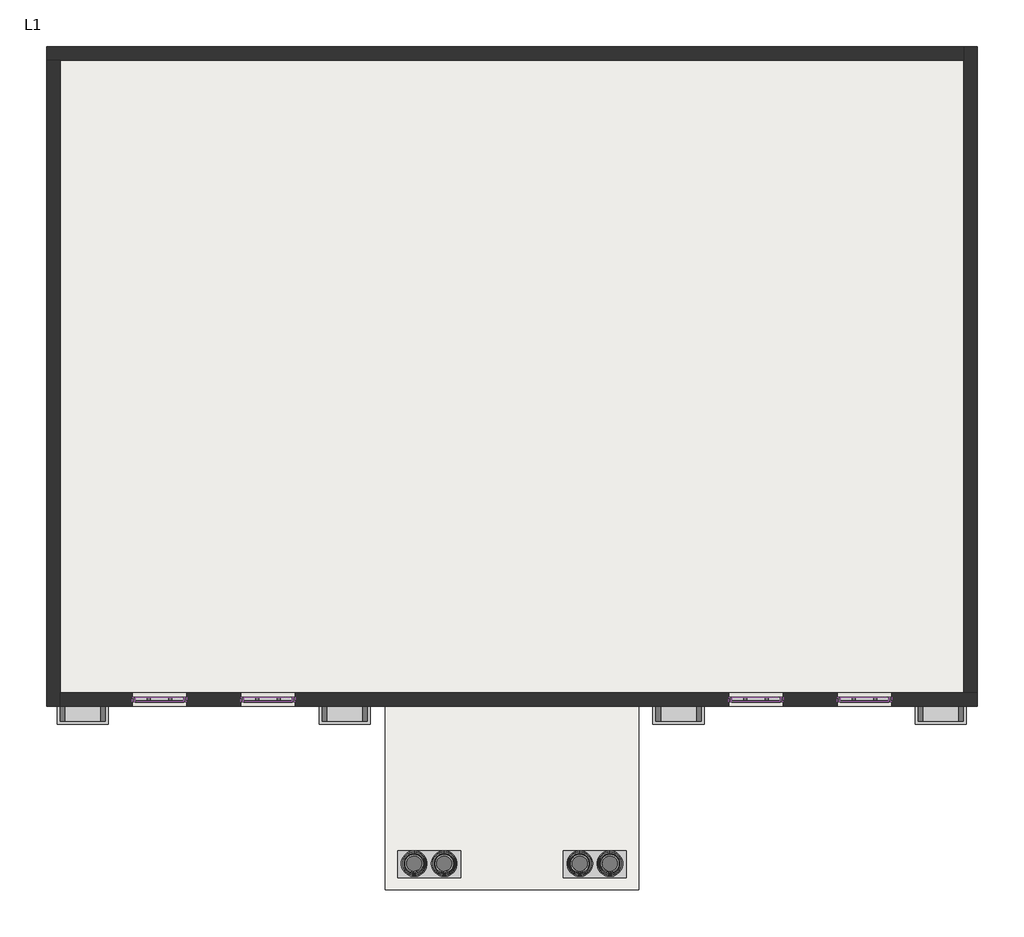
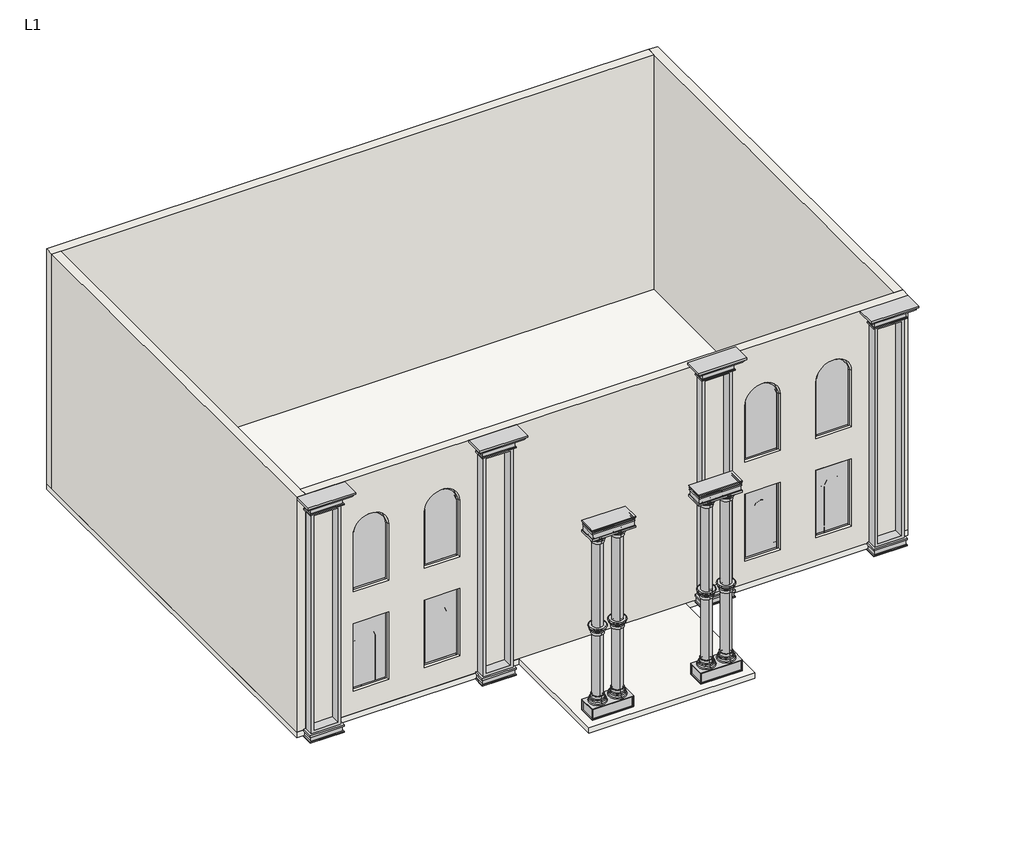
# One storey: 32 members, 10 proxies, 4 walls, 1 plate, 1 slab.
"""IFC4 building model written with IfcOpenShell, lengths in millimetres."""

from ifc_helpers import new_model, si_unit, frame, origin, place, context, project, spatial, polyline, circle_curve, outline, extrude, faceted_brep, transform, mapped, element, save
from ifc_brep_helpers import plane_surface, revolved_surface, advanced_brep
from components import generic_models_10_generic_models_9_50d809b8, generic_models_12_generic_models_12_08b21b51, generic_models_14_generic_models_14_9f9ef7df, generic_models_14_generic_models_14_a82bafd3, generic_models_14_generic_models_14_26f09abb, generic_models_5_generic_models_1_f7cfe2cb, member_492a078d, member_19d0c1c6, member_fb5b44a5, member_86f0261c, system_panel_glazed_d30904ce

model = new_model("IFC4")

# Units and contexts
model_context = context("Model", 3, world=origin())
ifc_project = project(units=[si_unit("LENGTHUNIT", "METRE", prefix="MILLI")], contexts=[model_context])

# Site, building, storey
site = spatial("IfcSite", under=ifc_project)
building = spatial("IfcBuilding", under=site)
storey = spatial("IfcBuildingStorey", under=building, Name="L1", Elevation=0.0)

# Proxies
placement = place(None, origin())
generic_models_10_generic_models_9_shape = generic_models_10_generic_models_9_50d809b8(model_context)
element("IfcBuildingElementProxy", 1, Name="Generic Models 10 : Generic Models 9", ObjectType="Generic Models 10 : Generic Models 9", at=placement, inside=storey, context=model_context, shape_type="MappedRepresentation", body=[
    mapped(generic_models_10_generic_models_9_shape, transform((14467.7065642, 0.0, 0.0), x_axis=(1.0, 0.0, 0.0), y_axis=(0.0, 1.0, 0.0), z_axis=(0.0, 0.0, 1.0))),
])
element("IfcBuildingElementProxy", 2, Name="Generic Models 11 : Generic Models 9", ObjectType="Generic Models 11 : Generic Models 9", at=placement, inside=storey, context=model_context, shape_type="MappedRepresentation", body=[
    mapped(generic_models_10_generic_models_9_shape, transform((4419.6, 0.0, 0.0), x_axis=(1.0, 0.0, 0.0), y_axis=(0.0, 1.0, 0.0), z_axis=(0.0, 0.0, 1.0))),
])
generic_models_12_generic_models_12_shape = generic_models_12_generic_models_12_08b21b51(model_context)
element("IfcBuildingElementProxy", 3, Name="Generic Models 12 : Generic Models 12", ObjectType="Generic Models 12 : Generic Models 12", at=placement, inside=storey, context=model_context, shape_type="MappedRepresentation", body=[
    mapped(generic_models_12_generic_models_12_shape, transform((0.0, 0.0, 0.0), x_axis=(1.0, 0.0, 0.0), y_axis=(0.0, 1.0, 0.0), z_axis=(0.0, 0.0, 1.0))),
])
element("IfcBuildingElementProxy", 4, Name="Generic Models 13 : Generic Models 9", ObjectType="Generic Models 13 : Generic Models 9", at=placement, inside=storey, context=model_context, shape_type="MappedRepresentation", body=[
    mapped(generic_models_10_generic_models_9_shape, transform((10048.1065642, 0.0, 138.370057), x_axis=(1.0, 0.0, 0.0), y_axis=(0.0, 1.0, 0.0), z_axis=(0.0, 0.0, 1.0))),
])
generic_models_14_generic_models_14_shape = generic_models_14_generic_models_14_9f9ef7df(model_context)
generic_models_14_generic_models_14_2_shape = generic_models_14_generic_models_14_a82bafd3(model_context)
generic_models_14_generic_models_14_3_shape = generic_models_14_generic_models_14_26f09abb(model_context)
element("IfcBuildingElementProxy", 5, Name="Generic Models 14 : Generic Models 14", ObjectType="Generic Models 14 : Generic Models 14", at=placement, inside=storey, context=model_context, shape_type="MappedRepresentation", body=[
    mapped(generic_models_14_generic_models_14_shape, transform((0.0, 0.0, 0.0), x_axis=(1.0, 0.0, 0.0), y_axis=(0.0, 1.0, 0.0), z_axis=(0.0, 0.0, 1.0))),
    mapped(generic_models_14_generic_models_14_2_shape, transform((0.0, 0.0, 0.0), x_axis=(1.0, 0.0, 0.0), y_axis=(0.0, 1.0, 0.0), z_axis=(0.0, 0.0, 1.0))),
    mapped(generic_models_14_generic_models_14_3_shape, transform((0.0, 0.0, 0.0), x_axis=(1.0, 0.0, 0.0), y_axis=(0.0, 1.0, 0.0), z_axis=(0.0, 0.0, 1.0))),
])
generic_models_5_generic_models_1_shape = generic_models_5_generic_models_1_f7cfe2cb(model_context)
element("IfcBuildingElementProxy", 6, Name="Generic Models 5 : Generic Models 1", ObjectType="Generic Models 5 : Generic Models 1", at=placement, inside=storey, context=model_context, shape_type="MappedRepresentation", body=[
    mapped(generic_models_5_generic_models_1_shape, transform((0.0, 0.0, 0.0), x_axis=(1.0, 0.0, 0.0), y_axis=(0.0, 1.0, 0.0), z_axis=(0.0, 0.0, 1.0))),
])
element("IfcBuildingElementProxy", 7, Name="Generic Models 6 : Generic Models 1", ObjectType="Generic Models 6 : Generic Models 1", at=placement, inside=storey, context=model_context, shape_type="MappedRepresentation", body=[
    mapped(generic_models_5_generic_models_1_shape, transform((1828.8, 0.0, 0.0), x_axis=(1.0, 0.0, 0.0), y_axis=(0.0, 1.0, 0.0), z_axis=(0.0, 0.0, 1.0))),
])
element("IfcBuildingElementProxy", 8, Name="Generic Models 7 : Generic Models 1", ObjectType="Generic Models 7 : Generic Models 1", at=placement, inside=storey, context=model_context, shape_type="MappedRepresentation", body=[
    mapped(generic_models_5_generic_models_1_shape, transform((10058.4, 0.0, 0.0), x_axis=(1.0, 0.0, 0.0), y_axis=(0.0, 1.0, 0.0), z_axis=(0.0, 0.0, 1.0))),
])
element("IfcBuildingElementProxy", 9, Name="Generic Models 8 : Generic Models 1", ObjectType="Generic Models 8 : Generic Models 1", at=placement, inside=storey, context=model_context, shape_type="MappedRepresentation", body=[
    mapped(generic_models_5_generic_models_1_shape, transform((11887.2, 0.0, 0.0), x_axis=(1.0, 0.0, 0.0), y_axis=(0.0, 1.0, 0.0), z_axis=(0.0, 0.0, 1.0))),
])
element("IfcBuildingElementProxy", 10, Name="Generic Models 9 : Generic Models 9", ObjectType="Generic Models 9 : Generic Models 9", at=placement, inside=storey, context=model_context, shape_type="MappedRepresentation", body=[
    mapped(generic_models_10_generic_models_9_shape, transform((0.0, 0.0, 0.0), x_axis=(1.0, 0.0, 0.0), y_axis=(0.0, 1.0, 0.0), z_axis=(0.0, 0.0, 1.0))),
])

# Members
member_shape = member_492a078d(model_context)
element("IfcMember", 11, ObjectType="Rectangular Mullion : 2.5\" x 5\" rectangular", at=placement, inside=storey, context=model_context, shape_type="MappedRepresentation", body=[
    mapped(member_shape, transform((-6449.8825076, -4772.1608295, 3302.0), x_axis=(0.0, 0.0, -1.0), y_axis=(0.0, 1.0, 0.0), z_axis=(1.0, 0.0, 0.0))),
])
element("IfcMember", 12, ObjectType="Rectangular Mullion : 2.5\" x 5\" rectangular", at=placement, inside=storey, context=model_context, shape_type="MappedRepresentation", body=[
    mapped(member_shape, transform((-6449.8825076, -4772.1608295, 609.6), x_axis=(0.0, 0.0, -1.0), y_axis=(0.0, 1.0, 0.0), z_axis=(1.0, 0.0, 0.0))),
])
element("IfcMember", 13, ObjectType="Rectangular Mullion : 2.5\" x 5\" rectangular", at=placement, inside=storey, context=model_context, shape_type="MappedRepresentation", body=[
    mapped(member_shape, transform((-4621.0825076, -4772.1608295, 3302.0), x_axis=(0.0, 0.0, -1.0), y_axis=(0.0, 1.0, 0.0), z_axis=(1.0, 0.0, 0.0))),
])
element("IfcMember", 14, ObjectType="Rectangular Mullion : 2.5\" x 5\" rectangular", at=placement, inside=storey, context=model_context, shape_type="MappedRepresentation", body=[
    mapped(member_shape, transform((-4621.0825076, -4772.1608295, 609.6), x_axis=(0.0, 0.0, -1.0), y_axis=(0.0, 1.0, 0.0), z_axis=(1.0, 0.0, 0.0))),
])
element("IfcMember", 15, ObjectType="Rectangular Mullion : 2.5\" x 5\" rectangular", at=placement, inside=storey, context=model_context, shape_type="MappedRepresentation", body=[
    mapped(member_shape, transform((3608.5174924, -4772.1608295, 3302.0), x_axis=(0.0, 0.0, -1.0), y_axis=(0.0, 1.0, 0.0), z_axis=(1.0, 0.0, 0.0))),
])
element("IfcMember", 16, ObjectType="Rectangular Mullion : 2.5\" x 5\" rectangular", at=placement, inside=storey, context=model_context, shape_type="MappedRepresentation", body=[
    mapped(member_shape, transform((3608.5174924, -4772.1608295, 609.6), x_axis=(0.0, 0.0, -1.0), y_axis=(0.0, 1.0, 0.0), z_axis=(1.0, 0.0, 0.0))),
])
element("IfcMember", 17, ObjectType="Rectangular Mullion : 2.5\" x 5\" rectangular", at=placement, inside=storey, context=model_context, shape_type="MappedRepresentation", body=[
    mapped(member_shape, transform((5437.3174924, -4772.1608295, 3302.0), x_axis=(0.0, 0.0, -1.0), y_axis=(0.0, 1.0, 0.0), z_axis=(1.0, 0.0, 0.0))),
])
element("IfcMember", 18, ObjectType="Rectangular Mullion : 2.5\" x 5\" rectangular", at=placement, inside=storey, context=model_context, shape_type="MappedRepresentation", body=[
    mapped(member_shape, transform((5437.3174924, -4772.1608295, 609.6), x_axis=(0.0, 0.0, -1.0), y_axis=(0.0, 1.0, 0.0), z_axis=(1.0, 0.0, 0.0))),
])
member_2_shape = member_19d0c1c6(model_context)
element("IfcMember", 19, ObjectType="Rectangular Mullion : 2.5\" x 5\" rectangular", at=placement, inside=storey, context=model_context, shape_type="MappedRepresentation", body=[
    mapped(member_2_shape, transform((-6399.0825076, -4772.1608295, 4826.0), x_axis=(1.0, 0.0, 0.0), y_axis=(0.0, 1.0, 0.0), z_axis=(0.0, 0.0, 1.0))),
])
element("IfcMember", 20, ObjectType="Rectangular Mullion : 2.5\" x 5\" rectangular", at=placement, inside=storey, context=model_context, shape_type="MappedRepresentation", body=[
    mapped(member_2_shape, transform((-4570.2825076, -4772.1608295, 4826.0), x_axis=(1.0, 0.0, 0.0), y_axis=(0.0, 1.0, 0.0), z_axis=(0.0, 0.0, 1.0))),
])
element("IfcMember", 21, ObjectType="Rectangular Mullion : 2.5\" x 5\" rectangular", at=placement, inside=storey, context=model_context, shape_type="MappedRepresentation", body=[
    mapped(member_2_shape, transform((3659.3174924, -4772.1608295, 4826.0), x_axis=(1.0, 0.0, 0.0), y_axis=(0.0, 1.0, 0.0), z_axis=(0.0, 0.0, 1.0))),
])
element("IfcMember", 22, ObjectType="Rectangular Mullion : 2.5\" x 5\" rectangular", at=placement, inside=storey, context=model_context, shape_type="MappedRepresentation", body=[
    mapped(member_2_shape, transform((5488.1174924, -4772.1608295, 4826.0), x_axis=(1.0, 0.0, 0.0), y_axis=(0.0, 1.0, 0.0), z_axis=(0.0, 0.0, 1.0))),
])
member_3_shape = member_fb5b44a5(model_context)
element("IfcMember", 23, ObjectType="Rectangular Mullion : 2.5\" x 5\" rectangular", at=placement, inside=storey, context=model_context, shape_type="MappedRepresentation", body=[
    mapped(member_3_shape, transform((-7313.4825076, -4772.1608295, 4826.0), x_axis=(-1.0, 0.0, 0.0), y_axis=(0.0, 1.0, 0.0), z_axis=(0.0, 0.0, -1.0))),
])
element("IfcMember", 24, ObjectType="Rectangular Mullion : 2.5\" x 5\" rectangular", at=placement, inside=storey, context=model_context, shape_type="MappedRepresentation", body=[
    mapped(member_3_shape, transform((-5484.6825076, -4772.1608295, 4826.0), x_axis=(-1.0, 0.0, 0.0), y_axis=(0.0, 1.0, 0.0), z_axis=(0.0, 0.0, -1.0))),
])
element("IfcMember", 25, ObjectType="Rectangular Mullion : 2.5\" x 5\" rectangular", at=placement, inside=storey, context=model_context, shape_type="MappedRepresentation", body=[
    mapped(member_3_shape, transform((2744.9174924, -4772.1608295, 4826.0), x_axis=(-1.0, 0.0, 0.0), y_axis=(0.0, 1.0, 0.0), z_axis=(0.0, 0.0, -1.0))),
])
element("IfcMember", 26, ObjectType="Rectangular Mullion : 2.5\" x 5\" rectangular", at=placement, inside=storey, context=model_context, shape_type="MappedRepresentation", body=[
    mapped(member_3_shape, transform((4573.7174924, -4772.1608295, 4826.0), x_axis=(-1.0, 0.0, 0.0), y_axis=(0.0, 1.0, 0.0), z_axis=(0.0, 0.0, -1.0))),
])
element("IfcMember", 27, ObjectType="Rectangular Mullion : 2.5\" x 5\" rectangular", at=placement, inside=storey, context=model_context, shape_type="MappedRepresentation", body=[
    mapped(member_shape, transform((-7262.6825076, -4772.1608295, 2438.4), x_axis=(0.0, 0.0, 1.0), y_axis=(0.0, 1.0, 0.0), z_axis=(-1.0, 0.0, 0.0))),
])
element("IfcMember", 28, ObjectType="Rectangular Mullion : 2.5\" x 5\" rectangular", at=placement, inside=storey, context=model_context, shape_type="MappedRepresentation", body=[
    mapped(member_shape, transform((-5433.8825076, -4772.1608295, 2438.4), x_axis=(0.0, 0.0, 1.0), y_axis=(0.0, 1.0, 0.0), z_axis=(-1.0, 0.0, 0.0))),
])
element("IfcMember", 29, ObjectType="Rectangular Mullion : 2.5\" x 5\" rectangular", at=placement, inside=storey, context=model_context, shape_type="MappedRepresentation", body=[
    mapped(member_shape, transform((2795.7174924, -4772.1608295, 2438.4), x_axis=(0.0, 0.0, 1.0), y_axis=(0.0, 1.0, 0.0), z_axis=(-1.0, 0.0, 0.0))),
])
element("IfcMember", 30, ObjectType="Rectangular Mullion : 2.5\" x 5\" rectangular", at=placement, inside=storey, context=model_context, shape_type="MappedRepresentation", body=[
    mapped(member_shape, transform((4624.5174924, -4772.1608295, 2438.4), x_axis=(0.0, 0.0, 1.0), y_axis=(0.0, 1.0, 0.0), z_axis=(-1.0, 0.0, 0.0))),
])
element("IfcMember", 31, ObjectType="Rectangular Mullion : 2.5\" x 5\" rectangular", at=placement, inside=storey, context=model_context, shape_type="MappedRepresentation", body=[
    mapped(member_2_shape, transform((-7313.4825076, -4772.1608295, 3302.0), x_axis=(-1.0, 0.0, 0.0), y_axis=(0.0, 1.0, 0.0), z_axis=(0.0, 0.0, -1.0))),
])
element("IfcMember", 32, ObjectType="Rectangular Mullion : 2.5\" x 5\" rectangular", at=placement, inside=storey, context=model_context, shape_type="MappedRepresentation", body=[
    mapped(member_2_shape, transform((-5484.6825076, -4772.1608295, 3302.0), x_axis=(-1.0, 0.0, 0.0), y_axis=(0.0, 1.0, 0.0), z_axis=(0.0, 0.0, -1.0))),
])
element("IfcMember", 33, ObjectType="Rectangular Mullion : 2.5\" x 5\" rectangular", at=placement, inside=storey, context=model_context, shape_type="MappedRepresentation", body=[
    mapped(member_2_shape, transform((2744.9174924, -4772.1608295, 3302.0), x_axis=(-1.0, 0.0, 0.0), y_axis=(0.0, 1.0, 0.0), z_axis=(0.0, 0.0, -1.0))),
])
element("IfcMember", 34, ObjectType="Rectangular Mullion : 2.5\" x 5\" rectangular", at=placement, inside=storey, context=model_context, shape_type="MappedRepresentation", body=[
    mapped(member_2_shape, transform((4573.7174924, -4772.1608295, 3302.0), x_axis=(-1.0, 0.0, 0.0), y_axis=(0.0, 1.0, 0.0), z_axis=(0.0, 0.0, -1.0))),
])
member_4_shape = member_86f0261c(model_context)
element("IfcMember", 35, ObjectType="Rectangular Mullion : 2.5\" x 5\" rectangular", at=placement, inside=storey, context=model_context, shape_type="MappedRepresentation", body=[
    mapped(member_4_shape, transform((-7313.4825076, -4772.1608295, 609.6), x_axis=(-1.0, 0.0, 0.0), y_axis=(0.0, 1.0, 0.0), z_axis=(0.0, 0.0, -1.0))),
])
element("IfcMember", 36, ObjectType="Rectangular Mullion : 2.5\" x 5\" rectangular", at=placement, inside=storey, context=model_context, shape_type="MappedRepresentation", body=[
    mapped(member_4_shape, transform((-5484.6825076, -4772.1608295, 609.6), x_axis=(-1.0, 0.0, 0.0), y_axis=(0.0, 1.0, 0.0), z_axis=(0.0, 0.0, -1.0))),
])
element("IfcMember", 37, ObjectType="Rectangular Mullion : 2.5\" x 5\" rectangular", at=placement, inside=storey, context=model_context, shape_type="MappedRepresentation", body=[
    mapped(member_4_shape, transform((2744.9174924, -4772.1608295, 609.6), x_axis=(-1.0, 0.0, 0.0), y_axis=(0.0, 1.0, 0.0), z_axis=(0.0, 0.0, -1.0))),
])
element("IfcMember", 38, ObjectType="Rectangular Mullion : 2.5\" x 5\" rectangular", at=placement, inside=storey, context=model_context, shape_type="MappedRepresentation", body=[
    mapped(member_4_shape, transform((4573.7174924, -4772.1608295, 609.6), x_axis=(-1.0, 0.0, 0.0), y_axis=(0.0, 1.0, 0.0), z_axis=(0.0, 0.0, -1.0))),
])
element("IfcMember", 39, ObjectType="Rectangular Mullion : 2.5\" x 5\" rectangular", at=placement, inside=storey, context=model_context, shape_type="MappedRepresentation", body=[
    mapped(member_4_shape, transform((-6399.0825076, -4772.1608295, 2438.4), x_axis=(1.0, 0.0, 0.0), y_axis=(0.0, 1.0, 0.0), z_axis=(0.0, 0.0, 1.0))),
])
element("IfcMember", 40, ObjectType="Rectangular Mullion : 2.5\" x 5\" rectangular", at=placement, inside=storey, context=model_context, shape_type="MappedRepresentation", body=[
    mapped(member_4_shape, transform((-4570.2825076, -4772.1608295, 2438.4), x_axis=(1.0, 0.0, 0.0), y_axis=(0.0, 1.0, 0.0), z_axis=(0.0, 0.0, 1.0))),
])
element("IfcMember", 41, ObjectType="Rectangular Mullion : 2.5\" x 5\" rectangular", at=placement, inside=storey, context=model_context, shape_type="MappedRepresentation", body=[
    mapped(member_4_shape, transform((3659.3174924, -4772.1608295, 2438.4), x_axis=(1.0, 0.0, 0.0), y_axis=(0.0, 1.0, 0.0), z_axis=(0.0, 0.0, 1.0))),
])
element("IfcMember", 42, ObjectType="Rectangular Mullion : 2.5\" x 5\" rectangular", at=placement, inside=storey, context=model_context, shape_type="MappedRepresentation", body=[
    mapped(member_4_shape, transform((5488.1174924, -4772.1608295, 2438.4), x_axis=(1.0, 0.0, 0.0), y_axis=(0.0, 1.0, 0.0), z_axis=(0.0, 0.0, 1.0))),
])

# Plate
system_panel_glazed_shape = system_panel_glazed_d30904ce(model_context)
element("IfcPlate", 43, ObjectType="System Panel : Glazed", at=placement, inside=storey, context=model_context, shape_type="MappedRepresentation", body=[
    mapped(system_panel_glazed_shape, transform((-912.6825076, -4772.1608295, 660.4), x_axis=(-1.0, 0.0, 0.0), y_axis=(0.0, -1.0, 0.0), z_axis=(0.0, 0.0, 1.0))),
])

# Slab
element("IfcSlab", 44, ObjectType="6\"", at=placement, inside=storey, context=model_context, shape_type="SweptSolid", body=[
    extrude(outline(polyline([(6935.9174924, 6238.7391705), (6935.9174924, -4886.4608295), (1220.9174924, -4886.4608295), (1220.9174924, -7983.4292912), (-3046.2825076, -7983.4292912), (-3046.2825076, -4886.4608295), (-8761.2825076, -4886.4608295), (-8761.2825076, 6238.7391705), (6935.9174924, 6238.7391705)])), frame((0.0, 0.0, -152.4), z_axis=(0.0, 0.0, 1.0), x_axis=(1.0, 0.0, 0.0)), (0.0, 0.0, 1.0), 152.4),
])

# Walls
element("IfcWall", 45, ObjectType="wall 9\"", at=placement, inside=storey, context=model_context, shape_type="Brep", body=[
    faceted_brep([(-8761.2825076, 6010.1391705, 0.0), (-8532.6825076, 6010.1391705, 0.0), (6707.3174924, 6010.1391705, 0.0), (6707.3174924, 6010.1391705, 6375.4), (-8532.6825076, 6010.1391705, 6375.4), (-8761.2825076, 6010.1391705, 6375.4), (-8761.2825076, 6238.7391705, 0.0), (-8761.2825076, 6238.7391705, 6375.4), (6707.3174924, 6238.7391705, 6375.4), (6707.3174924, 6238.7391705, 0.0)], [[[0, 1, 2, 3, 4, 5]], [[6, 7, 8, 9]], [[2, 1, 0, 6, 9]], [[0, 5, 7, 6]], [[3, 2, 9, 8]], [[5, 4, 3, 8, 7]]]),
])
element("IfcWall", 46, ObjectType="wall 9\"", at=placement, inside=storey, context=model_context, shape_type="Brep", body=[
    faceted_brep([(-8532.6825076, -4886.4608295, 0.0), (-8532.6825076, -4657.8608295, 0.0), (-8532.6825076, 6010.1391705, 0.0), (-8532.6825076, 6010.1391705, 6375.4), (-8532.6825076, -4657.8608295, 6375.4), (-8532.6825076, -4886.4608295, 6375.4), (-8761.2825076, -4886.4608295, 0.0), (-8761.2825076, -4886.4608295, 6375.4), (-8761.2825076, 6010.1391705, 6375.4), (-8761.2825076, 6010.1391705, 0.0)], [[[0, 1, 2, 3, 4, 5]], [[6, 7, 8, 9]], [[0, 5, 7, 6]], [[3, 2, 9, 8]], [[5, 4, 3, 8, 7]], [[2, 1, 0, 6, 9]]]),
])
element("IfcWall", 47, ObjectType="wall 9\"", at=placement, inside=storey, context=model_context, shape_type="AdvancedBrep", body=[
    advanced_brep(
    [(6935.9174924, -4657.8608295, 0.0), (6707.3174924, -4657.8608295, 0.0), (-8532.6825076, -4657.8608295, 0.0), (-8532.6825076, -4657.8608295, 6375.4), (6707.3174924, -4657.8608295, 6375.4), (6935.9174924, -4657.8608295, 6375.4), (-7313.4825076, -4657.8608295, 3302.0), (-6399.0825076, -4657.8608295, 3302.0), (-6399.0825076, -4657.8608295, 4826.0), (-7313.4825076, -4657.8608295, 4826.0), (-7313.4825076, -4657.8608295, 2438.4), (-7313.4825076, -4657.8608295, 609.6), (-6399.0825076, -4657.8608295, 609.6), (-6399.0825076, -4657.8608295, 2438.4), (-5484.6825076, -4657.8608295, 3302.0), (-4570.2825076, -4657.8608295, 3302.0), (-4570.2825076, -4657.8608295, 4826.0), (-5484.6825076, -4657.8608295, 4826.0), (-5484.6825076, -4657.8608295, 2438.4), (-5484.6825076, -4657.8608295, 609.6), (-4570.2825076, -4657.8608295, 609.6), (-4570.2825076, -4657.8608295, 2438.4), (5488.1174924, -4657.8608295, 3302.0), (5488.1174924, -4657.8608295, 4826.0), (4573.7174924, -4657.8608295, 4826.0), (4573.7174924, -4657.8608295, 3302.0), (5488.1174924, -4657.8608295, 2438.4), (4573.7174924, -4657.8608295, 2438.4), (4573.7174924, -4657.8608295, 609.6), (5488.1174924, -4657.8608295, 609.6), (3659.3174924, -4657.8608295, 3302.0), (3659.3174924, -4657.8608295, 4826.0), (2744.9174924, -4657.8608295, 4826.0), (2744.9174924, -4657.8608295, 3302.0), (3659.3174924, -4657.8608295, 2438.4), (2744.9174924, -4657.8608295, 2438.4), (2744.9174924, -4657.8608295, 609.6), (3659.3174924, -4657.8608295, 609.6), (6935.9174924, -4886.4608295, 0.0), (6935.9174924, -4886.4608295, 6375.4), (-8532.6825076, -4886.4608295, 6375.4), (-8532.6825076, -4886.4608295, 0.0), (-7313.4825076, -4886.4608295, 3302.0), (-7313.4825076, -4886.4608295, 4826.0), (-6399.0825076, -4886.4608295, 4826.0), (-6399.0825076, -4886.4608295, 3302.0), (-7313.4825076, -4886.4608295, 2438.4), (-6399.0825076, -4886.4608295, 2438.4), (-6399.0825076, -4886.4608295, 609.6), (-7313.4825076, -4886.4608295, 609.6), (-5484.6825076, -4886.4608295, 3302.0), (-5484.6825076, -4886.4608295, 4826.0), (-4570.2825076, -4886.4608295, 4826.0), (-4570.2825076, -4886.4608295, 3302.0), (-5484.6825076, -4886.4608295, 2438.4), (-4570.2825076, -4886.4608295, 2438.4), (-4570.2825076, -4886.4608295, 609.6), (-5484.6825076, -4886.4608295, 609.6), (5488.1174924, -4886.4608295, 3302.0), (4573.7174924, -4886.4608295, 3302.0), (4573.7174924, -4886.4608295, 4826.0), (5488.1174924, -4886.4608295, 4826.0), (5488.1174924, -4886.4608295, 2438.4), (5488.1174924, -4886.4608295, 609.6), (4573.7174924, -4886.4608295, 609.6), (4573.7174924, -4886.4608295, 2438.4), (3659.3174924, -4886.4608295, 3302.0), (2744.9174924, -4886.4608295, 3302.0), (2744.9174924, -4886.4608295, 4826.0), (3659.3174924, -4886.4608295, 4826.0), (3659.3174924, -4886.4608295, 2438.4), (3659.3174924, -4886.4608295, 609.6), (2744.9174924, -4886.4608295, 609.6), (2744.9174924, -4886.4608295, 2438.4)],
    [
        (0, 1),
        (1, 2),
        (2, 3),
        (3, 4),
        (4, 5),
        (5, 0),
        (6, 7),
        (7, 8),
        (8, 9, circle_curve(frame((-6856.2825076, -4657.8608295, 4826.0), z_axis=(0.0, -1.0, 0.0), x_axis=(1.0, 0.0, 0.0)), 457.2)),
        (9, 6),
        (10, 11),
        (11, 12),
        (12, 13),
        (13, 10),
        (14, 15),
        (15, 16),
        (16, 17, circle_curve(frame((-5027.4825076, -4657.8608295, 4826.0), z_axis=(0.0, -1.0, 0.0), x_axis=(1.0, 0.0, 0.0)), 457.2)),
        (17, 14),
        (18, 19),
        (19, 20),
        (20, 21),
        (21, 18),
        (22, 23),
        (23, 24, circle_curve(frame((5030.9174924, -4657.8608295, 4826.0), z_axis=(0.0, -1.0, 0.0), x_axis=(1.0, 0.0, 0.0)), 457.2)),
        (24, 25),
        (25, 22),
        (26, 27),
        (27, 28),
        (28, 29),
        (29, 26),
        (30, 31),
        (31, 32, circle_curve(frame((3202.1174924, -4657.8608295, 4826.0), z_axis=(0.0, -1.0, 0.0), x_axis=(1.0, 0.0, 0.0)), 457.2)),
        (32, 33),
        (33, 30),
        (34, 35),
        (35, 36),
        (36, 37),
        (37, 34),
        (38, 39),
        (39, 40),
        (40, 41),
        (41, 38),
        (42, 43),
        (43, 44, circle_curve(frame((-6856.2825076, -4886.4608295, 4826.0), z_axis=(0.0, 1.0, 0.0), x_axis=(1.0, 0.0, 0.0)), 457.2)),
        (44, 45),
        (45, 42),
        (46, 47),
        (47, 48),
        (48, 49),
        (49, 46),
        (50, 51),
        (51, 52, circle_curve(frame((-5027.4825076, -4886.4608295, 4826.0), z_axis=(0.0, 1.0, 0.0), x_axis=(1.0, 0.0, 0.0)), 457.2)),
        (52, 53),
        (53, 50),
        (54, 55),
        (55, 56),
        (56, 57),
        (57, 54),
        (58, 59),
        (59, 60),
        (60, 61, circle_curve(frame((5030.9174924, -4886.4608295, 4826.0), z_axis=(0.0, 1.0, 0.0), x_axis=(1.0, 0.0, 0.0)), 457.2)),
        (61, 58),
        (62, 63),
        (63, 64),
        (64, 65),
        (65, 62),
        (66, 67),
        (67, 68),
        (68, 69, circle_curve(frame((3202.1174924, -4886.4608295, 4826.0), z_axis=(0.0, 1.0, 0.0), x_axis=(1.0, 0.0, 0.0)), 457.2)),
        (69, 66),
        (70, 71),
        (71, 72),
        (72, 73),
        (73, 70),
        (5, 39),
        (38, 0),
        (2, 41),
        (40, 3),
        (6, 42),
        (45, 7),
        (44, 8),
        (43, 9),
        (10, 46),
        (49, 11),
        (48, 12),
        (47, 13),
        (14, 50),
        (53, 15),
        (52, 16),
        (51, 17),
        (18, 54),
        (57, 19),
        (56, 20),
        (55, 21),
        (22, 58),
        (61, 23),
        (60, 24),
        (59, 25),
        (26, 62),
        (65, 27),
        (64, 28),
        (63, 29),
        (30, 66),
        (69, 31),
        (68, 32),
        (67, 33),
        (34, 70),
        (73, 35),
        (72, 36),
        (71, 37),
    ],
    [
        plane_surface(frame((5602.4174924, -4657.8608295, 0.0), z_axis=(0.0, 1.0, 0.0), x_axis=(-1.0, 0.0, 0.0))),
        plane_surface(frame((5602.4174924, -4886.4608295, 0.0), z_axis=(0.0, -1.0, 0.0), x_axis=(1.0, 0.0, 0.0))),
        plane_surface(frame((6935.9174924, 15954.2391705, 0.0), z_axis=(1.0, 0.0, 0.0), x_axis=(0.0, 1.0, 0.0))),
        plane_surface(frame((-8532.6825076, 14735.0391705, 0.0), z_axis=(-1.0, 0.0, 0.0), x_axis=(0.0, 1.0, 0.0))),
        plane_surface(frame((6821.6174924, -4657.8608295, 0.0), z_axis=(0.0, 0.0, -1.0), x_axis=(0.0, -1.0, 0.0))),
        plane_surface(frame((-7313.4825076, -4657.8608295, 3302.0), z_axis=(0.0, 0.0, 1.0), x_axis=(0.0, -1.0, 0.0))),
        plane_surface(frame((-6399.0825076, -4657.8608295, 3302.0), z_axis=(-1.0, 0.0, 0.0), x_axis=(0.0, -1.0, 0.0))),
        revolved_surface(polyline([(-6399.0825076, -4886.4608295, 4826.0), (-6399.0825076, -4657.8608295, 4826.0)]), (-6856.2825076, -4772.1608295, 4826.0), (0.0, -1.0, 0.0)),
        plane_surface(frame((-7313.4825076, -4657.8608295, 4826.0), z_axis=(1.0, 0.0, 0.0), x_axis=(0.0, -1.0, 0.0))),
        plane_surface(frame((-7313.4825076, -4657.8608295, 2438.4), z_axis=(1.0, 0.0, 0.0), x_axis=(0.0, -1.0, 0.0))),
        plane_surface(frame((-7313.4825076, -4657.8608295, 609.6), z_axis=(0.0, 0.0, 1.0), x_axis=(0.0, -1.0, 0.0))),
        plane_surface(frame((-6399.0825076, -4657.8608295, 609.6), z_axis=(-1.0, 0.0, 0.0), x_axis=(0.0, -1.0, 0.0))),
        plane_surface(frame((-6399.0825076, -4657.8608295, 2438.4), z_axis=(0.0, 0.0, -1.0), x_axis=(0.0, -1.0, 0.0))),
        plane_surface(frame((-5484.6825076, -4657.8608295, 3302.0), z_axis=(0.0, 0.0, 1.0), x_axis=(0.0, -1.0, 0.0))),
        plane_surface(frame((-4570.2825076, -4657.8608295, 3302.0), z_axis=(-1.0, 0.0, 0.0), x_axis=(0.0, -1.0, 0.0))),
        revolved_surface(polyline([(-4570.2825076, -4886.4608295, 4826.0), (-4570.2825076, -4657.8608295, 4826.0)]), (-5027.4825076, -4772.1608295, 4826.0), (0.0, -1.0, 0.0)),
        plane_surface(frame((-5484.6825076, -4657.8608295, 4826.0), z_axis=(1.0, 0.0, 0.0), x_axis=(0.0, -1.0, 0.0))),
        plane_surface(frame((-5484.6825076, -4657.8608295, 2438.4), z_axis=(1.0, 0.0, 0.0), x_axis=(0.0, -1.0, 0.0))),
        plane_surface(frame((-5484.6825076, -4657.8608295, 609.6), z_axis=(0.0, 0.0, 1.0), x_axis=(0.0, -1.0, 0.0))),
        plane_surface(frame((-4570.2825076, -4657.8608295, 609.6), z_axis=(-1.0, 0.0, 0.0), x_axis=(0.0, -1.0, 0.0))),
        plane_surface(frame((-4570.2825076, -4657.8608295, 2438.4), z_axis=(0.0, 0.0, -1.0), x_axis=(0.0, -1.0, 0.0))),
        plane_surface(frame((5488.1174924, -4657.8608295, 3302.0), z_axis=(-1.0, 0.0, 0.0), x_axis=(0.0, -1.0, 0.0))),
        revolved_surface(polyline([(5488.1174924, -4886.4608295, 4826.0), (5488.1174924, -4657.8608295, 4826.0)]), (5030.9174924, -4772.1608295, 4826.0), (0.0, -1.0, 0.0)),
        plane_surface(frame((4573.7174924, -4657.8608295, 4826.0), z_axis=(1.0, 0.0, 0.0), x_axis=(0.0, -1.0, 0.0))),
        plane_surface(frame((4573.7174924, -4657.8608295, 3302.0), z_axis=(0.0, 0.0, 1.0), x_axis=(0.0, -1.0, 0.0))),
        plane_surface(frame((5488.1174924, -4657.8608295, 2438.4), z_axis=(0.0, 0.0, -1.0), x_axis=(0.0, -1.0, 0.0))),
        plane_surface(frame((4573.7174924, -4657.8608295, 2438.4), z_axis=(1.0, 0.0, 0.0), x_axis=(0.0, -1.0, 0.0))),
        plane_surface(frame((4573.7174924, -4657.8608295, 609.6), z_axis=(0.0, 0.0, 1.0), x_axis=(0.0, -1.0, 0.0))),
        plane_surface(frame((5488.1174924, -4657.8608295, 609.6), z_axis=(-1.0, 0.0, 0.0), x_axis=(0.0, -1.0, 0.0))),
        plane_surface(frame((3659.3174924, -4657.8608295, 3302.0), z_axis=(-1.0, 0.0, 0.0), x_axis=(0.0, -1.0, 0.0))),
        revolved_surface(polyline([(3659.3174924, -4886.4608295, 4826.0), (3659.3174924, -4657.8608295, 4826.0)]), (3202.1174924, -4772.1608295, 4826.0), (0.0, -1.0, 0.0)),
        plane_surface(frame((2744.9174924, -4657.8608295, 4826.0), z_axis=(1.0, 0.0, 0.0), x_axis=(0.0, -1.0, 0.0))),
        plane_surface(frame((2744.9174924, -4657.8608295, 3302.0), z_axis=(0.0, 0.0, 1.0), x_axis=(0.0, -1.0, 0.0))),
        plane_surface(frame((3659.3174924, -4657.8608295, 2438.4), z_axis=(0.0, 0.0, -1.0), x_axis=(0.0, -1.0, 0.0))),
        plane_surface(frame((2744.9174924, -4657.8608295, 2438.4), z_axis=(1.0, 0.0, 0.0), x_axis=(0.0, -1.0, 0.0))),
        plane_surface(frame((2744.9174924, -4657.8608295, 609.6), z_axis=(0.0, 0.0, 1.0), x_axis=(0.0, -1.0, 0.0))),
        plane_surface(frame((3659.3174924, -4657.8608295, 609.6), z_axis=(-1.0, 0.0, 0.0), x_axis=(0.0, -1.0, 0.0))),
        plane_surface(frame((6935.9174924, 6238.7391705, 6375.4), z_axis=(0.0, 0.0, 1.0), x_axis=(0.0, -1.0, 0.0))),
    ],
    [
        (0, [[1, 2, 3, 4, 5, 6], [7, 8, 9, 10], [11, 12, 13, 14], [15, 16, 17, 18], [19, 20, 21, 22], [23, 24, 25, 26], [27, 28, 29, 30], [31, 32, 33, 34], [35, 36, 37, 38]]),
        (1, [[39, 40, 41, 42], [43, 44, 45, 46], [47, 48, 49, 50], [51, 52, 53, 54], [55, 56, 57, 58], [59, 60, 61, 62], [63, 64, 65, 66], [67, 68, 69, 70], [71, 72, 73, 74]]),
        (2, [[-6, 75, -39, 76]]),
        (3, [[-3, 77, -41, 78]]),
        (4, [[-2, -1, -76, -42, -77]]),
        (5, [[-7, 79, -46, 80]]),
        (6, [[-8, -80, -45, 81]]),
        (7, [[-9, -81, -44, 82]]),
        (8, [[-10, -82, -43, -79]]),
        (9, [[-11, 83, -50, 84]]),
        (10, [[-12, -84, -49, 85]]),
        (11, [[-13, -85, -48, 86]]),
        (12, [[-14, -86, -47, -83]]),
        (13, [[-15, 87, -54, 88]]),
        (14, [[-16, -88, -53, 89]]),
        (15, [[-17, -89, -52, 90]]),
        (16, [[-18, -90, -51, -87]]),
        (17, [[-19, 91, -58, 92]]),
        (18, [[-20, -92, -57, 93]]),
        (19, [[-21, -93, -56, 94]]),
        (20, [[-22, -94, -55, -91]]),
        (21, [[-23, 95, -62, 96]]),
        (22, [[-24, -96, -61, 97]]),
        (23, [[-25, -97, -60, 98]]),
        (24, [[-26, -98, -59, -95]]),
        (25, [[-27, 99, -66, 100]]),
        (26, [[-28, -100, -65, 101]]),
        (27, [[-29, -101, -64, 102]]),
        (28, [[-30, -102, -63, -99]]),
        (29, [[-31, 103, -70, 104]]),
        (30, [[-32, -104, -69, 105]]),
        (31, [[-33, -105, -68, 106]]),
        (32, [[-34, -106, -67, -103]]),
        (33, [[-35, 107, -74, 108]]),
        (34, [[-36, -108, -73, 109]]),
        (35, [[-37, -109, -72, 110]]),
        (36, [[-38, -110, -71, -107]]),
        (37, [[-5, -4, -78, -40, -75]]),
    ],
),
])
element("IfcWall", 48, ObjectType="wall 9\"", at=placement, inside=storey, context=model_context, shape_type="Brep", body=[
    faceted_brep([(6707.3174924, 6238.7391705, 0.0), (6707.3174924, 6010.1391705, 0.0), (6707.3174924, -4657.8608295, 0.0), (6707.3174924, -4657.8608295, 6375.4), (6707.3174924, 6010.1391705, 6375.4), (6707.3174924, 6238.7391705, 6375.4), (6935.9174924, 6238.7391705, 0.0), (6935.9174924, 6238.7391705, 6375.4), (6935.9174924, -4657.8608295, 6375.4), (6935.9174924, -4657.8608295, 0.0)], [[[0, 1, 2, 3, 4, 5]], [[6, 7, 8, 9]], [[2, 1, 0, 6, 9]], [[0, 5, 7, 6]], [[3, 2, 9, 8]], [[5, 4, 3, 8, 7]]]),
])

save(model, "model.ifc")

# Revit data of these elements
# Type "Rectangular Mullion : 2.5\" x 5\" rectangular"
#   built-in parameter 1007304 = 0.25 (stored number, unit not read)
#   built-in parameter 1007301 = 0.0833333 (stored number, unit not read)
#   built-in parameter 1007300 = 0.0833333 (stored number, unit not read)
# Type "System Panel : Glazed"
#   Construction Type Id = "GSP4R"
#   Analytic Construction = "1/8 in Pilkington single glazing"
#   Visual Light Transmittance = 0.9
#   Solar Heat Gain Coefficient = 0.86
#   Heat Transfer Coefficient (U) = 1.18115 BTU/(h·ft²·°F)
#   Define Thermal Properties by = 1
# Type "6\""
#   Description = "Generic Floor (Material By Category), 12\" thick"
#   Assembly Code = "B1010"
#   Type Mark = "G01"
#   Function = 0
#   Layers, outside or top first: 0' - 6" no material (function 1)
# Type "wall 9\""
#   Description = "Generic Wall (Material By Category), 8\" thick"
#   Assembly Code = "B2010"
#   Type Mark = "G06"
#   Layers, outside or top first: 0' - 9" no material (function 1)
# Element 1 (IfcBuildingElementProxy, "Generic Models 10 : Generic Models 9")
#   Phase Created = New Construction
# Element 2 (IfcBuildingElementProxy, "Generic Models 11 : Generic Models 9")
#   Phase Created = New Construction
# Element 3 (IfcBuildingElementProxy, "Generic Models 12 : Generic Models 12")
#   Phase Created = New Construction
# Element 4 (IfcBuildingElementProxy, "Generic Models 13 : Generic Models 9")
#   Phase Created = New Construction
# Element 5 (IfcBuildingElementProxy, "Generic Models 14 : Generic Models 14")
#   Phase Created = New Construction
# Element 6 (IfcBuildingElementProxy, "Generic Models 5 : Generic Models 1")
#   Phase Created = New Construction
#   Materials on its faces: "Aluminum"
# Element 7 (IfcBuildingElementProxy, "Generic Models 6 : Generic Models 1")
#   Phase Created = New Construction
#   Materials on its faces: "Aluminum"
# Element 8 (IfcBuildingElementProxy, "Generic Models 7 : Generic Models 1")
#   Phase Created = New Construction
#   Materials on its faces: "Aluminum"
# Element 9 (IfcBuildingElementProxy, "Generic Models 8 : Generic Models 1")
#   Phase Created = New Construction
#   Materials on its faces: "Aluminum"
# Element 10 (IfcBuildingElementProxy, "Generic Models 9 : Generic Models 9")
#   Phase Created = New Construction
# Elements 11, 12, 13, 14, 15, 16, 17, 18, 19, 20, 21, 22, 23, 24, 25, 26, 27, 28, 29, 30, 31, 32, 33, 34, 35, 36, 37, 38, 39, 40, 41, 42 (IfcMember, "Rectangular Mullion : 2.5\" x 5\" rectangular")
#   Phase Created = New Construction
#   Materials on its faces: "Aluminum"
# Element 43 (IfcPlate, "System Panel : Glazed")
#   Phase Created = New Construction
#   Materials on its faces: "Glass"
# Element 44 (IfcSlab, "6\"")
#   Height Offset From Level = 0' - 0"
#   Phase Created = New Construction
#   Materials on its faces: "Default Floor"
# Elements 45, 46, 47, 48 (IfcWall, "wall 9\"")
#   Top Offset = 0' - 0"
#   Base Offset = 0' - 0"
#   wall height = 20' - 11"
#   Phase Created = New Construction
#   Base Constraint = L1
#   Top Constraint = L3
#   Materials on its faces: "Default Wall"
# Materials
#   "Aluminum": class "Metal", colour RGB 244 245 246, transparency 0, Description = "Aluminum 6061", Cost = 0
#   "Glass": class "Glass", colour RGB 245 245 243, transparency 1, Description = "Soda Lime Glass", Cost = 0
#   "Default Floor": colour RGB 128 128 128, transparency 0, Cost = 0
#   "Default Wall": colour RGB 192 192 192, transparency 0, Cost = 0
